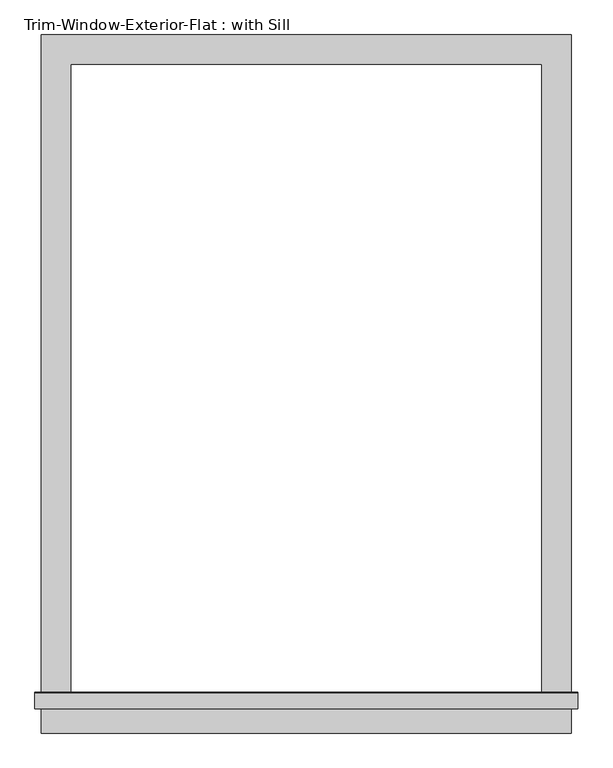
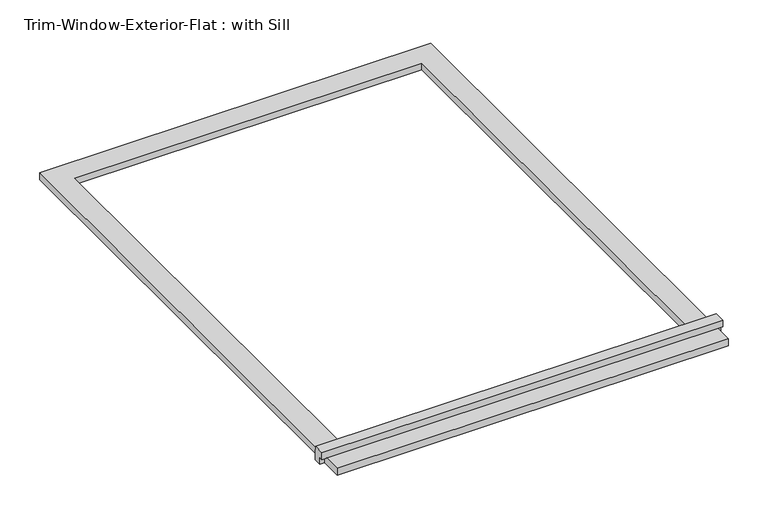
"""IFC4 building model written with IfcOpenShell, lengths in millimetres: proxy geometry, Trim-Window-Exterior-Flat : with Sill."""

from ifc_helpers import new_model, si_unit, frame, origin, origin_with_axes, place, context, project, spatial, polyline, outline, extrude, source, transform, mapped, element, save


def trim_window_exterior_flat_with_sill_e4b28ec3(model_context):
    return source(origin(), model_context, "Body", "SweptSolid", [
        extrude(outline(polyline([(514.35, -1241.3823709), (514.35, -1298.5323709), (-514.35, -1298.5323709), (-514.35, -1241.3823709), (514.35, -1241.3823709)])), origin_with_axes(), (0.0, 0.0, 1.0), 19.05),
        extrude(outline(polyline([(-1250.95, 38.1), (-1221.6580645, 38.1), (-1219.2, 19.05), (-1219.2, 0.0), (-1241.3823709, 0.0), (-1241.3823709, 19.05), (-1250.95, 19.05), (-1250.95, 38.1)])), frame((-527.05, 0.0, 0.0), z_axis=(1.0, 0.0, 0.0), x_axis=(0.0, 1.0, 0.0)), (0.0, 0.0, 1.0), 1054.1),
        extrude(outline(polyline([(-514.35, 57.15), (514.35, 57.15), (514.35, -1219.2), (457.2, -1219.2), (457.2, 0.0), (-457.2, 0.0), (-457.2, -1219.2), (-514.35, -1219.2), (-514.35, 57.15)])), origin_with_axes(), (0.0, 0.0, 1.0), 19.05),
    ])


if __name__ == "__main__":
    model = new_model("IFC4")
    model_context = context("Model", 3, world=origin())
    ifc_project = project(units=[si_unit("LENGTHUNIT", "METRE", prefix="MILLI")], contexts=[model_context])
    site = spatial("IfcSite", under=ifc_project)
    building = spatial("IfcBuilding", under=site)
    placement = place(None, origin())
    trim_window_exterior_flat_with_sill_shape = trim_window_exterior_flat_with_sill_e4b28ec3(model_context)
    element("IfcBuildingElementProxy", 1, Name="Trim-Window-Exterior-Flat : with Sill", ObjectType="Trim-Window-Exterior-Flat : with Sill", at=placement, inside=building, context=model_context, shape_type="MappedRepresentation", body=[
        mapped(trim_window_exterior_flat_with_sill_shape, transform((0.0, 0.0, 0.0), x_axis=(1.0, 0.0, 0.0), y_axis=(0.0, 1.0, 0.0), z_axis=(0.0, 0.0, 1.0))),
    ])
    save(model, "model.ifc")

# Revit data of these elements
# Type "Trim-Window-Exterior-Flat : with Sill"
#   Trim Width = 0' - 2 1/4"
#   Trim Thickness_Picture Frame = 0' - 1 1/4"
#   Trim Thickness_with Sill = 0' - 0 3/4"
#   Sill Thickness = 0' - 1 1/4"
#   Opening Width [instance default] = 2' - 0"
#   Opening Height [instance default] = 3' - 0"
#   Default Elevation = 4' - 0"
#   Sill = yes
#   Picture Frame = no
#   Trim Material [instance default] = none
# Element 1 (IfcBuildingElementProxy, "Trim-Window-Exterior-Flat : with Sill")
#   Opening Width = 3' - 0"
#   Opening Height = 4' - 0"
#   Trim Material = Clad - White
#   Materials on its faces: "Clad - White"
# Materials
#   "Clad - White": class "Wood", colour RGB 245 245 243, transparency 0, Cost = 0
